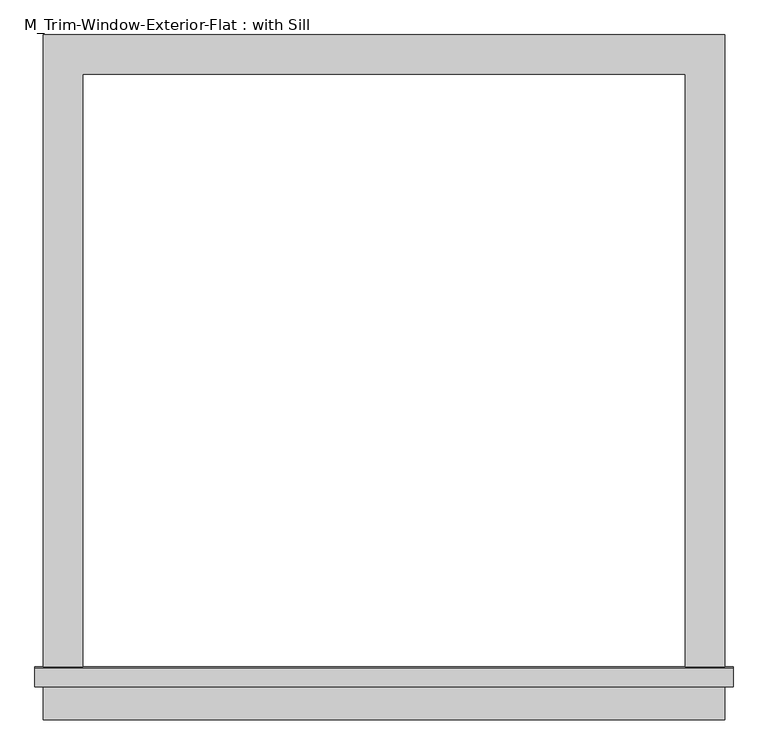
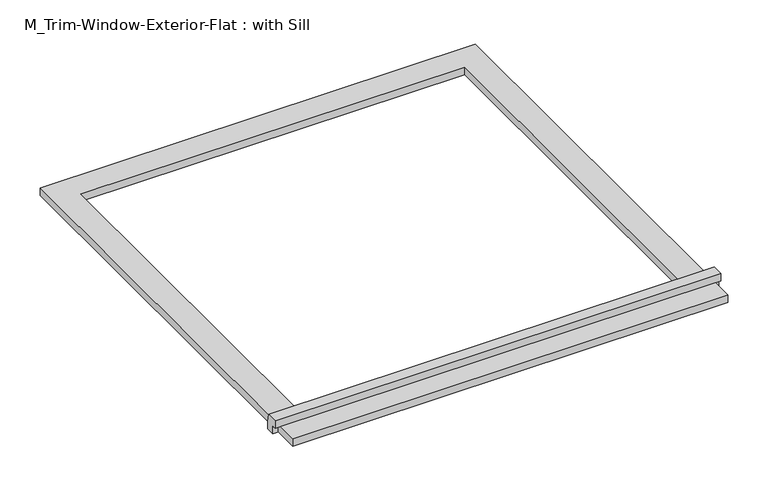
"""IFC4 building model written with IfcOpenShell, lengths in millimetres: proxy geometry, M_Trim-Window-Exterior-Flat : with Sill."""

from ifc_helpers import new_model, si_unit, frame, origin, origin_with_axes, place, context, project, spatial, polyline, outline, extrude, source, transform, mapped, element, save


def m_trim_window_exterior_flat_with_sill_8fa486dc(model_context):
    return source(origin(), model_context, "Body", "SweptSolid", [
        extrude(outline(polyline([(517.2, -920.4323709), (517.2, -980.4323709), (-517.2, -980.4323709), (-517.2, -920.4323709), (517.2, -920.4323709)])), origin_with_axes(), (0.0, 0.0, 1.0), 19.05),
        extrude(outline(polyline([(-930.0, 38.1), (-902.4580645, 38.1), (-900.0, 19.05), (-900.0, 0.0), (-920.4323709, 0.0), (-920.4323709, 19.05), (-930.0, 19.05), (-930.0, 38.1)])), frame((-529.9, 0.0, 0.0), z_axis=(1.0, 0.0, 0.0), x_axis=(0.0, 1.0, 0.0)), (0.0, 0.0, 1.0), 1059.8),
        extrude(outline(polyline([(-517.2, 60.0), (517.2, 60.0), (517.2, -900.0), (457.2, -900.0), (457.2, 0.0), (-457.2, 0.0), (-457.2, -900.0), (-517.2, -900.0), (-517.2, 60.0)])), origin_with_axes(), (0.0, 0.0, 1.0), 19.05),
    ])


if __name__ == "__main__":
    model = new_model("IFC4")
    model_context = context("Model", 3, world=origin())
    ifc_project = project(units=[si_unit("LENGTHUNIT", "METRE", prefix="MILLI")], contexts=[model_context])
    site = spatial("IfcSite", under=ifc_project)
    building = spatial("IfcBuilding", under=site)
    placement = place(None, origin())
    m_trim_window_exterior_flat_with_sill_shape = m_trim_window_exterior_flat_with_sill_8fa486dc(model_context)
    element("IfcBuildingElementProxy", 1, Name="M_Trim-Window-Exterior-Flat : with Sill", ObjectType="M_Trim-Window-Exterior-Flat : with Sill", at=placement, inside=building, context=model_context, shape_type="MappedRepresentation", body=[
        mapped(m_trim_window_exterior_flat_with_sill_shape, transform((0.0, 0.0, 0.0), x_axis=(1.0, 0.0, 0.0), y_axis=(0.0, 1.0, 0.0), z_axis=(0.0, 0.0, 1.0))),
    ])
    save(model, "model.ifc")

# Revit data of these elements
# Type "M_Trim-Window-Exterior-Flat : with Sill"
#   Trim Width = 0' - 2.3622"
#   Trim Thickness_Picture Frame = 0' - 1.1811"
#   Trim Thickness_with Sill = 0' - 0 3/4"
#   Sill Thickness = 0' - 1.1811"
#   Opening Width [instance default] = 1' - 11.62205"
#   Opening Height [instance default] = 2' - 11.43307"
#   Default Elevation = 3' - 11.24409"
#   Sill = yes
#   Picture Frame = no
#   Trim Material [instance default] = none
# Element 1 (IfcBuildingElementProxy, "M_Trim-Window-Exterior-Flat : with Sill")
#   Opening Width = 3' - 0"
#   Trim Material = Clad - White
#   Materials on its faces: "Clad - White"
# Materials
#   "Clad - White": class "Wood", colour RGB 242 242 238, transparency 0, Cost = 0
